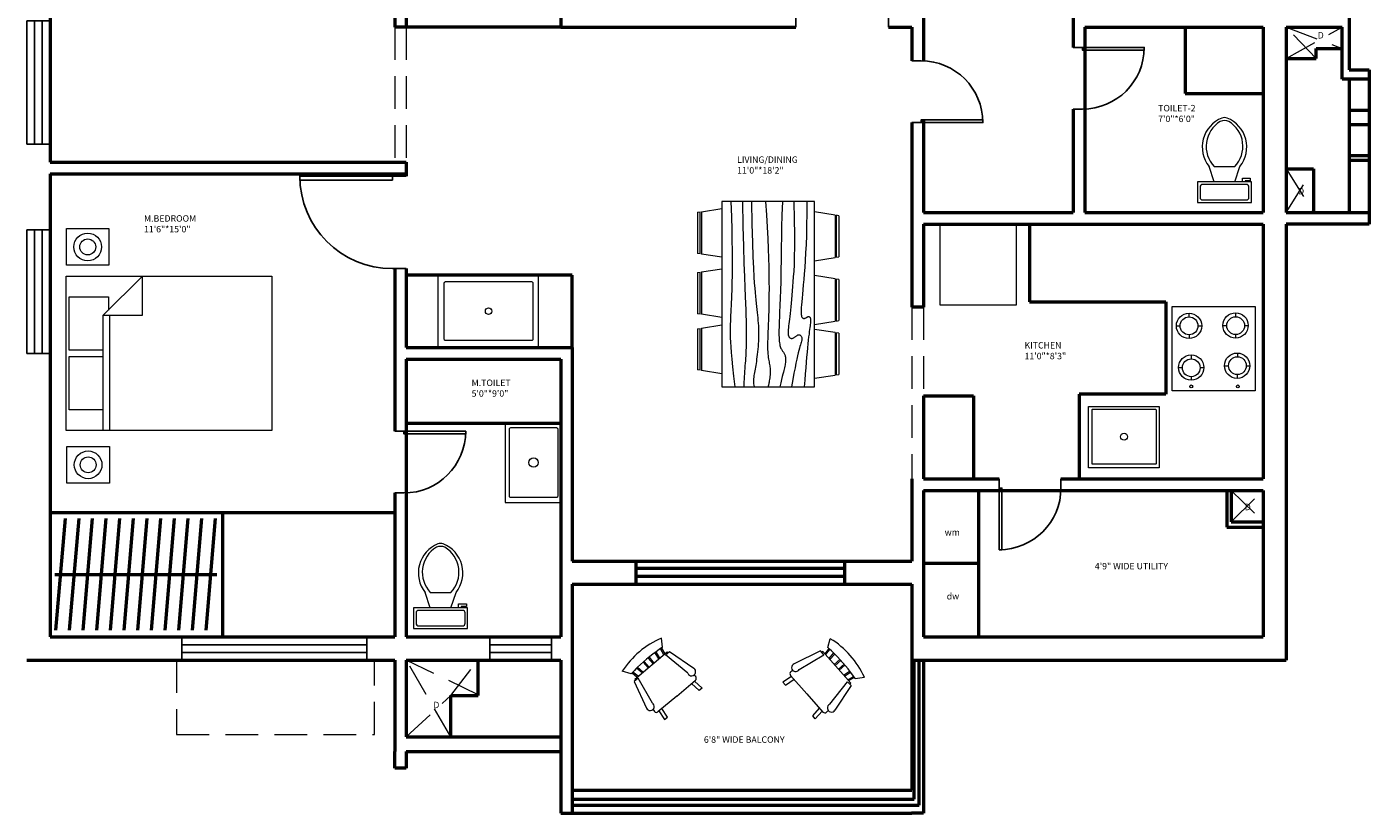
# Model space of a CAD drawing. Units: inches. Extents: x 291 to 2631, y 456 to 2623.
# Tile 10 of 22: x 2109 to 2631, y 468 to 774. Entities that reach past the tile are written whole.
import ezdxf

# ---------------------------------------------------------------- set-up
doc = ezdxf.new("R2010")
doc.units = ezdxf.units.IN
doc.linetypes.add('DASHED', pattern=[19.05, 12.7, -6.35])
for name, color, linetype, lineweight in [('A-ANNO-TEXT', 3, 'Continuous', 25), ('A-AREA-IDEN', 7, 'Continuous', 25), ('A-DOOR', 3, 'Continuous', 25), ('A-EQPM', 8, 'Continuous', 18), ('A-FLOR-FIXT', 9, 'Continuous', 18), ('A-FLOR-OVHD', 1, 'DASHED', 18), ('A-FURN', 8, 'Continuous', 18), ('A-GLAZ', 4, 'Continuous', 25), ('A-WALL', 7, 'Continuous', 50)]:
    doc.layers.add(name, color=color, linetype=linetype, lineweight=lineweight)
doc.styles.get("Standard").update_dxf_attribs({"font": 'arial.ttf'})

# ---------------------------------------------------------------- blocks, each defined once
blk = doc.blocks.new('*U2')
for p, q in [((0, 0), (0, -6)), ((40, 0), (40, -6))]:
    blk.add_line(p, q)
blk.add_lwpolyline([(0, 0), (0, 40), (1.75, 40), (1.75, 0)], close=True)
blk.add_arc((0, 0), 40, 0, 90)
blk = doc.blocks.new('Toilet - top')
for p, q in [((9.5, -6), (9.5, -2)), ((-10, -8.5), (-8, -8.5)), ((-10, -9.5), (-10, -8.5)), ((-7, -9.5), (-10, -9.5)), ((-8, -8.5), (-8, -8)), ((-7, -8), (-7, -9.5)), ((-4, -8), (-6, -14)), ((4, -8), (6, -14)), ((4, -14), (-4, -14))]:
    blk.add_line(p, q)
blk.add_lwpolyline([(10.5, -8), (10.5, 0), (-10.5, 0), (-10.5, -8)], close=True)
for points in [[(-9.5, -2), (-9.5, -6)], [(8.5, -1), (-8.5, -1)], [(-8.5, -7), (8.5, -7)]]:
    blk.add_lwpolyline(points)
for centre, radius, start, end in [((-8.62, -1.88), 0.884, 81.8699, 188.1301), ((8.62, -1.88), 0.884, 351.8699, 98.1301), ((-8.62, -6.12), 0.884, 171.8699, 278.1301), ((8.62, -6.12), 0.884, 261.8699, 8.1301), ((3.52, -21.58), 12.17, 141.4691, 247.9714), ((4.2, -21.82), 11.33, 136.3677, 238.9468), ((-3.52, -21.58), 12.17, 292.0284, 38.5307), ((-4.2, -21.82), 11.33, 301.053, 43.6321), ((0, -27.88), 4, 245.7318, 294.2682), ((0, -29), 4, 254.8605, 285.1395)]:
    blk.add_arc(centre, radius, start, end)
blk = doc.blocks.new('Bed - Queen')
for p, q in [((0, -80.00003), (0, 0)), ((0, 0), (59.99999, 0)), ((59.99999, 0), (59.99999, -80.00003)), ((7.99999, -1.2), (28.79998, -1.2)), ((7.99999, -14.4), (7.99999, -1.2)), ((28.79998, -1.2), (28.79998, -14.4)), ((31.19999, -1.2), (51.99999, -1.2)), ((31.19999, -14.4), (31.19999, -1.2)), ((51.99999, -1.2), (51.99999, -16.4)), ((0, -14.4), (44.8, -14.4)), ((59.99999, -29.6), (44.8, -14.4)), ((44.8, -14.4), (44.8, -29.6)), ((44.8, -16.8), (0, -16.8)), ((51.99999, -16.4), (46.79936, -16.4)), ((44.8, -29.6), (59.99999, -29.6)), ((59.99999, -80.00003), (0, -80.00003))]:
    blk.add_line(p, q)
blk = doc.blocks.new('Chair - Rocking')
for p, q in [((-8, -4.5), (-10, -1.5)), ((-7.5, -4.5), (-7, -7)), ((-6.5, -7), (-7.02225, -4.43)), ((-4.5, -7), (-4.96674, -4.19951)), ((-4, -7), (-4.40532, -4.16272)), ((-1.5, -4.05012), (-1.5, -7)), ((-1, -7), (-1, -4.05012)), ((1, -7), (1, -4.04655)), ((1.5, -4.05012), (1.5, -7)), ((4, -7), (4.40187, -4.18694)), ((4.5, -7), (4.96761, -4.19437)), ((6.5, -7), (7, -4.4057)), ((7.5, -4.5), (7, -7)), ((8, -4.5), (10, -1.5)), ((-9, -7.5), (-12, -18.49999)), ((-7, -7.5), (-9, -7.5)), ((-9, -18.49999), (-7, -7.5)), ((-8.23428, -6.99939), (-8.3093, -7.47958)), ((-8.23041, -7), (8.23915, -7)), ((7, -7.5), (9, -7.5)), ((9, -18.49999), (7, -7.5)), ((8.31071, -7.48854), (8.23449, -7.00073)), ((9, -7.5), (12, -18.49999)), ((-10.36644, -20.64523), (-10.5, -21.49999)), ((10.5, -21.49999), (10.3575, -20.58798)), ((-9, -22.49999), (-9.5, -26.49999)), ((0, -22.49999), (-9.5, -22.49999)), ((-8, -26.49999), (-7.5, -22.49999)), ((0, -22.49999), (9.5, -22.49999)), ((8, -26.49999), (7.5, -22.49999)), ((9, -22.49999), (9.5, -26.49999)), ((-9.5, -26.49999), (-8, -26.49999)), ((9.5, -26.49999), (8, -26.49999))]:
    blk.add_line(p, q)
for centre, radius, start, end in [((0, -34.08333), 34.08333, 72.93847, 107.0615), ((0, -68.25004), 64.25, 93.92211, 97.15267), ((0, -68.25004), 64.25, 82.84733, 93.92211), ((-10.5, -18.99999), 1.58114, 161.5651, 18.43495), ((10.5, -18.99999), 1.58114, 161.5651, 18.43495), ((-9.5, -21.49999), 1, 180, 270), ((9.5, -21.49999), 1, 270, 0)]:
    blk.add_arc(centre, radius, start, end)
blk = doc.blocks.new('WIN-1800')
for p, q in [((0, 9), (72, 9)), ((0, 0), (0, 9)), ((0, 6), (72, 6)), ((72, 9), (72, 0)), ((72, 3), (0, 3)), ((72, 0), (0, 0))]:
    blk.add_line(p, q)
blk = doc.blocks.new('WIN-1200')
for p, q in [((0, 0), (0, 48)), ((0, 48), (9, 48)), ((3, 0), (3, 48)), ((6, 48), (6, 0)), ((9, 48), (9, 0)), ((9, 0), (0, 0))]:
    blk.add_line(p, q)
blk = doc.blocks.new('COOKTOP')
for p, q in [((6.54, 28.68), (6.54, 30.14)), ((24.62, 30.31), (24.62, 28.76)), ((1.62, 25.22), (3.08, 25.22)), ((6.54, 21.76), (6.54, 20.3)), ((10, 25.22), (11.46, 25.22)), ((19.7, 25.39), (21.21, 25.39)), ((24.62, 21.83), (24.62, 20.47)), ((28.13, 25.39), (29.54, 25.39)), ((7.38, 13.92), (7.38, 12.38)), ((25.35, 14.65), (25.34, 13.21)), ((2.46, 9), (3.95, 9)), ((7.38, 5.46), (7.38, 4.08)), ((10.87, 9), (12.3, 9)), ((20.32, 9.73), (21.89, 9.73)), ((25.26, 6.28), (25.24, 4.81)), ((28.81, 9.73), (30.16, 9.73))]:
    blk.add_line(p, q)
blk.add_lwpolyline([(0, 32.79), (32.25, 32.79), (32.25, 0), (0, 0)], close=True)
for centre, radius in [((6.54, 25.22), 4.92), ((6.54, 25.22), 3.46), ((24.62, 25.39), 4.92), ((24.67, 25.29), 3.46), ((7.38, 9), 4.92), ((7.41, 8.92), 3.46), ((25.24, 9.73), 4.92), ((25.35, 9.74), 3.46), ((7.38, 1.69), 0.572), ((25.5, 1.69), 0.572)]:
    blk.add_circle(centre, radius)
blk = doc.blocks.new('WIN-600')
for p, q in [((24, 9), (0, 9)), ((0, 9), (0, 0)), ((24, 6), (0, 6)), ((24, 0), (24, 9)), ((0, 3), (24, 3)), ((0, 0), (24, 0))]:
    blk.add_line(p, q)

msp = doc.modelspace()

# ---------------------------------------------------------------- linework, layer by layer
at = {"layer": 'A-FLOR-OVHD'}
for p, q in [((2251.97, 773.48), (2251.97, 720.98)), ((2256.47, 773.48), (2256.47, 720.98)), ((2598.47, 773.48), (2620.18, 765.26)), ((2598.47, 761.4), (2620.18, 773.48)), ((2610.19, 761.4), (2598.47, 773.48)), ((2598.47, 718.48), (2609.11, 701.48)), ((2598.47, 701.48), (2609.11, 718.48)), ((2452.97, 664.67), (2452.97, 597.98)), ((2457.47, 664.67), (2457.47, 630.2)), ((2577.06, 593.48), (2589.47, 581.26)), ((2577.06, 581.26), (2589.47, 593.48)), ((2167.17, 527.48), (2167.17, 498.51)), ((2244.14, 498.51), (2244.14, 527.48)), ((2273.76, 497.61), (2256.47, 527.48)), ((2284.38, 514), (2256.47, 527.48)), ((2273.76, 513.73), (2284.38, 527.48)), ((2256.47, 497.61), (2273.76, 513.73)), ((2167.17, 498.51), (2244.14, 498.51))]:
    msp.add_line(p, q, dxfattribs=at)
at = {"layer": 'A-FURN'}
for p, q in [((2379.15, 705.74), (2379.15, 633.74)), ((2415.15, 705.74), (2379.15, 705.74)), ((2415.15, 633.74), (2415.15, 705.74)), ((2369.65, 701.56), (2370.65, 701.71)), ((2369.65, 701.56), (2369.65, 685.56)), ((2370.65, 685.4), (2370.65, 701.71)), ((2371.15, 701.79), (2379.15, 703.04)), ((2371.15, 701.79), (2371.15, 685.32)), ((2423.15, 700.46), (2415.15, 701.71)), ((2423.15, 700.45), (2423.15, 683.98)), ((2424.65, 700.22), (2423.65, 700.38)), ((2423.65, 684.06), (2423.65, 700.37)), ((2424.65, 700.22), (2424.65, 684.22)), ((2370.65, 685.4), (2369.65, 685.56)), ((2379.15, 684.07), (2371.15, 685.32)), ((2415.15, 682.74), (2423.15, 683.99)), ((2423.65, 684.07), (2424.65, 684.22)), ((2369.65, 678.15), (2370.65, 678.3)), ((2370.65, 661.99), (2370.65, 678.3)), ((2371.15, 678.38), (2379.15, 679.63)), ((2371.15, 678.38), (2371.15, 661.91)), ((2369.65, 678.15), (2369.65, 662.15)), ((2423.15, 675.68), (2415.15, 676.93)), ((2423.15, 675.67), (2423.15, 659.2)), ((2424.65, 675.44), (2423.65, 675.6)), ((2423.65, 659.28), (2423.65, 675.59)), ((2424.65, 675.44), (2424.65, 659.44)), ((2370.65, 661.99), (2369.65, 662.15)), ((2379.15, 660.66), (2371.15, 661.91)), ((2371.15, 656.53), (2379.15, 657.78)), ((2415.15, 657.96), (2423.15, 659.21)), ((2423.65, 659.28), (2424.65, 659.44)), ((2369.65, 656.3), (2370.65, 656.45)), ((2369.65, 656.3), (2369.65, 640.3)), ((2370.65, 640.14), (2370.65, 656.45)), ((2371.15, 656.53), (2371.15, 640.06)), ((2423.15, 654.77), (2415.15, 656.02)), ((2423.15, 654.77), (2423.15, 638.3)), ((2424.65, 654.54), (2423.65, 654.69)), ((2423.65, 638.38), (2423.65, 654.69)), ((2424.65, 654.54), (2424.65, 638.54)), ((2370.65, 640.14), (2369.65, 640.3)), ((2379.15, 638.81), (2371.15, 640.06)), ((2415.15, 637.05), (2423.15, 638.3)), ((2423.65, 638.38), (2424.65, 638.54)), ((2379.15, 633.74), (2415.15, 633.74))]:
    msp.add_line(p, q, dxfattribs=at)
for points in [[(2382.65, 705.74), (2382.82, 699.83), (2382.94, 694.78), (2383.02, 690.48), (2383.08, 686.82), (2383.1, 683.71), (2383.11, 681.05), (2383.09, 678.72), (2383.07, 676.62), (2383.03, 674.67), (2382.99, 672.84), (2382.94, 671.12), (2382.89, 669.5), (2382.83, 667.98), (2382.78, 666.55), (2382.71, 665.19), (2382.65, 663.91), (2382.59, 662.69), (2382.53, 661.51), (2382.47, 660.35), (2382.43, 659.2), (2382.39, 658.03), (2382.36, 656.82), (2382.35, 655.55), (2382.36, 654.2), (2382.39, 652.75), (2382.45, 651.13), (2382.55, 649.26), (2382.71, 647.08), (2382.94, 644.51), (2383.24, 641.48), (2383.65, 637.92), (2384.15, 633.74)], [(2387.15, 705.74), (2387.34, 696.15), (2387.52, 688.21), (2387.7, 681.73), (2387.87, 676.48), (2388.03, 672.27), (2388.17, 668.87), (2388.3, 666.07), (2388.4, 663.66), (2388.48, 661.47), (2388.54, 659.44), (2388.59, 657.57), (2388.61, 655.85), (2388.62, 654.26), (2388.61, 652.79), (2388.59, 651.42), (2388.57, 650.16), (2388.53, 648.98), (2388.49, 647.88), (2388.44, 646.83), (2388.39, 645.82), (2388.32, 644.84), (2388.26, 643.87), (2388.19, 642.9), (2388.11, 641.91), (2388.03, 640.9), (2387.95, 639.86), (2387.87, 638.81), (2387.8, 637.77), (2387.74, 636.72), (2387.69, 635.7), (2387.66, 634.7), (2387.65, 633.74)], [(2390.65, 705.74), (2390.84, 696.93), (2391.03, 689.83), (2391.21, 684.21), (2391.39, 679.85), (2391.57, 676.52), (2391.74, 673.98), (2391.91, 672.01), (2392.07, 670.37), (2392.22, 668.87), (2392.36, 667.47), (2392.5, 666.16), (2392.63, 664.92), (2392.75, 663.74), (2392.86, 662.62), (2392.97, 661.54), (2393.07, 660.49), (2393.16, 659.47), (2393.24, 658.47), (2393.31, 657.48), (2393.36, 656.49), (2393.4, 655.51), (2393.42, 654.52), (2393.42, 653.52), (2393.4, 652.49), (2393.36, 651.45), (2393.3, 650.4), (2393.22, 649.34), (2393.12, 648.3), (2393.01, 647.27), (2392.9, 646.27), (2392.78, 645.32), (2392.65, 644.41), (2392.53, 643.57), (2392.4, 642.78), (2392.28, 642.03), (2392.16, 641.32), (2392.04, 640.64), (2391.92, 639.99), (2391.8, 639.34), (2391.69, 638.7), (2391.59, 638.06), (2391.49, 637.42), (2391.42, 636.78), (2391.38, 636.15), (2391.37, 635.52), (2391.41, 634.91), (2391.5, 634.32), (2391.65, 633.74)], [(2396.15, 705.74), (2396.49, 700.54), (2396.77, 695.76), (2396.99, 691.4), (2397.16, 687.4), (2397.28, 683.75), (2397.36, 680.4), (2397.42, 677.32), (2397.44, 674.49), (2397.45, 671.88), (2397.44, 669.46), (2397.41, 667.21), (2397.38, 665.13), (2397.33, 663.19), (2397.27, 661.38), (2397.21, 659.68), (2397.15, 658.08), (2397.09, 656.55), (2397.03, 655.11), (2396.98, 653.75), (2396.93, 652.46), (2396.9, 651.26), (2396.88, 650.14), (2396.88, 649.11), (2396.9, 648.16), (2396.94, 647.3), (2397.01, 646.51), (2397.08, 645.79), (2397.17, 645.13), (2397.27, 644.52), (2397.37, 643.95), (2397.47, 643.42), (2397.57, 642.91), (2397.66, 642.42), (2397.74, 641.93), (2397.81, 641.46), (2397.86, 640.97), (2397.9, 640.48), (2397.92, 639.98), (2397.92, 639.46), (2397.9, 638.91), (2397.86, 638.34), (2397.8, 637.75), (2397.72, 637.16), (2397.64, 636.58), (2397.55, 636.04), (2397.47, 635.55), (2397.39, 635.13), (2397.32, 634.79), (2397.26, 634.53), (2397.22, 634.36), (2397.19, 634.24), (2397.17, 634.16), (2397.16, 634.09), (2397.15, 634.01), (2397.15, 633.9), (2397.15, 633.74)], [(2402.65, 705.74), (2402.49, 700.46), (2402.36, 695.81), (2402.27, 691.74), (2402.2, 688.17), (2402.16, 685.05), (2402.12, 682.3), (2402.1, 679.86), (2402.07, 677.66), (2402.03, 675.65), (2401.99, 673.8), (2401.94, 672.09), (2401.89, 670.48), (2401.83, 668.97), (2401.78, 667.52), (2401.71, 666.12), (2401.65, 664.74), (2401.59, 663.37), (2401.53, 662.01), (2401.47, 660.67), (2401.42, 659.37), (2401.38, 658.11), (2401.35, 656.92), (2401.33, 655.79), (2401.32, 654.74), (2401.33, 653.79), (2401.35, 652.93), (2401.39, 652.14), (2401.44, 651.44), (2401.51, 650.81), (2401.6, 650.26), (2401.7, 649.76), (2401.82, 649.33), (2401.95, 648.95), (2402.1, 648.61), (2402.25, 648.32), (2402.41, 648.06), (2402.58, 647.82), (2402.74, 647.59), (2402.91, 647.38), (2403.07, 647.16), (2403.22, 646.94), (2403.36, 646.7), (2403.49, 646.46), (2403.61, 646.19), (2403.71, 645.91), (2403.79, 645.6), (2403.86, 645.27), (2403.9, 644.91), (2403.92, 644.52), (2403.92, 644.1), (2403.89, 643.66), (2403.85, 643.19), (2403.78, 642.71), (2403.7, 642.2), (2403.6, 641.69), (2403.48, 641.16), (2403.35, 640.62), (2403.2, 640.04), (2403.02, 639.38), (2402.82, 638.61), (2402.58, 637.7), (2402.31, 636.6), (2402, 635.3), (2401.65, 633.74)], [(2407.15, 705.74), (2407.29, 698.72), (2407.36, 692.92), (2407.35, 688.17), (2407.29, 684.31), (2407.18, 681.18), (2407.05, 678.62), (2406.89, 676.46), (2406.73, 674.54), (2406.58, 672.71), (2406.44, 670.97), (2406.3, 669.3), (2406.16, 667.72), (2406.03, 666.22), (2405.9, 664.8), (2405.78, 663.48), (2405.65, 662.24), (2405.53, 661.1), (2405.41, 660.05), (2405.29, 659.09), (2405.18, 658.21), (2405.09, 657.42), (2405.01, 656.7), (2404.94, 656.06), (2404.9, 655.49), (2404.88, 655), (2404.88, 654.56), (2404.91, 654.19), (2404.95, 653.87), (2405.02, 653.6), (2405.1, 653.36), (2405.2, 653.16), (2405.32, 652.99), (2405.45, 652.85), (2405.6, 652.73), (2405.75, 652.64), (2405.92, 652.57), (2406.1, 652.53), (2406.28, 652.51), (2406.46, 652.53), (2406.65, 652.58), (2406.84, 652.66), (2407.03, 652.76), (2407.21, 652.88), (2407.4, 653.02), (2407.59, 653.16), (2407.78, 653.3), (2407.96, 653.45), (2408.15, 653.58), (2408.34, 653.69), (2408.53, 653.79), (2408.71, 653.87), (2408.89, 653.92), (2409.07, 653.95), (2409.24, 653.94), (2409.41, 653.9), (2409.57, 653.83), (2409.72, 653.72), (2409.86, 653.57), (2409.98, 653.38), (2410.09, 653.17), (2410.17, 652.93), (2410.22, 652.67), (2410.25, 652.38), (2410.23, 652.08), (2410.18, 651.76), (2410.1, 651.4), (2409.98, 651.01), (2409.83, 650.55), (2409.66, 650.03), (2409.47, 649.41), (2409.25, 648.7), (2409.03, 647.87), (2408.78, 646.91), (2408.52, 645.79), (2408.24, 644.47), (2407.92, 642.92), (2407.56, 641.1), (2407.15, 638.99), (2406.68, 636.55), (2406.15, 633.74)], [(2412.15, 705.74), (2412.13, 700.92), (2412.07, 696.55), (2411.97, 692.6), (2411.84, 689.02), (2411.69, 685.78), (2411.52, 682.84), (2411.34, 680.16), (2411.15, 677.7), (2410.96, 675.43), (2410.78, 673.35), (2410.61, 671.44), (2410.44, 669.71), (2410.3, 668.15), (2410.17, 666.76), (2410.06, 665.55), (2409.98, 664.49), (2409.94, 663.61), (2409.92, 662.86), (2409.93, 662.26), (2409.96, 661.77), (2410.02, 661.38), (2410.1, 661.07), (2410.2, 660.84), (2410.32, 660.66), (2410.45, 660.52), (2410.6, 660.42), (2410.75, 660.36), (2410.91, 660.32), (2411.08, 660.31), (2411.24, 660.32), (2411.41, 660.36), (2411.57, 660.41), (2411.72, 660.48), (2411.87, 660.56), (2412.01, 660.65), (2412.14, 660.73), (2412.27, 660.82), (2412.4, 660.89), (2412.53, 660.95), (2412.65, 660.99), (2412.78, 661.01), (2412.9, 661.01), (2413.02, 660.98), (2413.13, 660.93), (2413.24, 660.86), (2413.33, 660.76), (2413.41, 660.64), (2413.48, 660.49), (2413.54, 660.33), (2413.58, 660.13), (2413.6, 659.89), (2413.61, 659.62), (2413.6, 659.3), (2413.58, 658.92), (2413.54, 658.49), (2413.48, 657.99), (2413.41, 657.43), (2413.33, 656.78), (2413.23, 656.03), (2413.12, 655.18), (2413, 654.21), (2412.86, 653.1), (2412.72, 651.86), (2412.57, 650.45), (2412.41, 648.89), (2412.24, 647.16), (2412.07, 645.27), (2411.89, 643.24), (2411.71, 641.06), (2411.53, 638.75), (2411.34, 636.31), (2411.15, 633.74)]]:
    msp.add_lwpolyline(points, dxfattribs=at)
for points in [[(2124.4, 695.25), (2140.88, 695.25), (2140.88, 680.95), (2124.4, 680.95)], [(2464.03, 696.98), (2493.54, 696.98), (2493.54, 665.42), (2464.03, 665.42)], [(2268.91, 677.11), (2307.71, 677.11), (2307.71, 648.98), (2268.91, 648.98)], [(2521.67, 626.1), (2549.11, 626.1), (2549.11, 602.2), (2521.67, 602.2)], [(2316.47, 619.55), (2294.95, 619.55), (2294.95, 588.8), (2316.47, 588.8)], [(2124.55, 610.55), (2141.04, 610.55), (2141.04, 596.25), (2124.55, 596.25)]]:
    msp.add_lwpolyline(points, close=True, dxfattribs=at)
for points in [[(2271.72, 674.6), (2305.19, 674.6, -0.414214), (2305.69, 674.1), (2305.69, 652.2, -0.414214), (2305.19, 651.7), (2271.72, 651.7, -0.414214), (2271.22, 652.2), (2271.22, 674.1, -0.414214)], [(2523.31, 624.99), (2547.61, 624.99, -0.414214), (2547.91, 624.69), (2547.91, 603.91, -0.414214), (2547.61, 603.61), (2523.31, 603.61, -0.414214), (2523.01, 603.91), (2523.01, 624.69, -0.414214)], [(2297.06, 617.84), (2314.83, 617.84, -0.414214), (2315.33, 617.34), (2315.33, 591.15, -0.414214), (2314.83, 590.65), (2297.06, 590.65, -0.414214), (2296.56, 591.15), (2296.56, 617.34, -0.414214)]]:
    msp.add_lwpolyline(points, format="xyb", close=True, dxfattribs=at)
for centre, radius in [((2132.64, 688.1), 5.39), ((2132.64, 688.1), 3.08), ((2288.46, 663.15), 1.27), ((2535.46, 614.3), 1.36), ((2132.79, 603.4), 5.39), ((2132.79, 603.4), 3.08), ((2305.94, 604.25), 1.82)]:
    msp.add_circle(centre, radius, dxfattribs=at)
at = {"layer": 'A-WALL'}
for p, q in [((2117.97, 921.98), (2117.97, 720.98)), ((2251.97, 921.98), (2251.97, 773.48)), ((2457.47, 921.98), (2457.47, 773.48)), ((2256.47, 809.48), (2256.47, 773.48)), ((2316.47, 809.48), (2316.47, 773.48)), ((2515.69, 777.98), (2515.69, 765.67)), ((2622.9, 779.28), (2622.9, 756.88)), ((2316.47, 773.48), (2251.97, 773.48)), ((2316.47, 773.48), (2407.89, 773.48)), ((2443.89, 773.48), (2452.97, 773.48)), ((2452.97, 773.48), (2452.97, 760.44)), ((2457.47, 773.48), (2457.47, 760.42)), ((2520.19, 773.48), (2520.19, 701.48)), ((2520.19, 773.48), (2589.47, 773.48)), ((2559.17, 773.48), (2559.17, 747.73)), ((2589.47, 773.48), (2589.47, 701.48)), ((2598.47, 773.48), (2620.18, 773.48)), ((2598.47, 773.48), (2598.47, 701.48)), ((2620.18, 756.88), (2620.18, 773.48)), ((2610.19, 761.4), (2610.19, 765.26)), ((2610.19, 765.26), (2620.18, 765.26)), ((2598.47, 761.4), (2610.19, 761.4)), ((2620.18, 753.26), (2620.18, 756.88)), ((2622.9, 756.88), (2630.73, 756.88)), ((2630.73, 756.88), (2630.73, 753.26)), ((2622.9, 753.26), (2620.18, 753.26)), ((2630.73, 753.26), (2622.9, 753.26)), ((2622.9, 753.26), (2622.9, 701.48)), ((2630.73, 753.26), (2630.73, 696.98)), ((2559.17, 747.73), (2589.47, 747.73)), ((2515.69, 741.67), (2515.69, 701.48)), ((2622.9, 741.23), (2622.9, 741.23)), ((2622.9, 741.23), (2630.73, 741.23)), ((2452.97, 736.44), (2452.97, 664.67)), ((2457.47, 737.49), (2457.47, 701.48)), ((2622.9, 735.75), (2630.73, 735.75)), ((2117.97, 720.98), (2256.47, 720.98)), ((2256.47, 720.98), (2256.47, 715.66)), ((2622.9, 723.68), (2630.73, 723.68)), ((2622.9, 721.88), (2630.73, 721.88)), ((2117.97, 716.48), (2256.47, 716.48)), ((2117.97, 716.48), (2117.97, 536.48)), ((2251.97, 716.48), (2251.97, 715.66)), ((2598.47, 718.48), (2609.11, 718.48)), ((2609.11, 718.48), (2609.11, 701.48)), ((2457.47, 701.48), (2515.69, 701.48)), ((2520.19, 701.48), (2589.47, 701.48)), ((2598.47, 701.48), (2630.73, 701.48)), ((2457.47, 696.98), (2589.47, 696.98)), ((2457.47, 696.98), (2457.47, 664.67)), ((2498.71, 696.98), (2498.71, 666.81)), ((2589.47, 696.98), (2589.47, 597.98)), ((2622.9, 696.98), (2598.47, 696.98)), ((2598.47, 696.98), (2598.47, 527.48)), ((2630.73, 696.98), (2622.9, 696.98)), ((2251.97, 679.66), (2251.97, 616.47)), ((2256.47, 679.66), (2256.47, 648.98)), ((2320.97, 677.11), (2256.47, 677.11)), ((2320.97, 648.98), (2320.97, 677.11)), ((2457.47, 664.67), (2452.97, 664.67)), ((2498.71, 666.81), (2551.69, 666.81)), ((2551.69, 666.81), (2551.69, 630.86)), ((2256.47, 648.98), (2320.97, 648.98)), ((2320.97, 648.98), (2320.97, 565.99)), ((2256.47, 644.48), (2316.47, 644.48)), ((2256.47, 644.48), (2256.47, 536.48)), ((2316.47, 644.48), (2316.47, 536.48)), ((2457.47, 630.2), (2476.96, 630.2)), ((2457.47, 630.2), (2457.47, 597.98)), ((2476.96, 630.2), (2476.96, 597.98)), ((2551.69, 630.86), (2518.04, 630.86)), ((2518.04, 630.86), (2518.04, 597.98)), ((2256.47, 619.55), (2316.47, 619.55)), ((2452.97, 597.98), (2452.97, 565.99)), ((2457.47, 597.98), (2486.93, 597.98)), ((2510.93, 597.98), (2589.47, 597.98)), ((2251.97, 592.47), (2251.97, 536.48)), ((2457.47, 593.48), (2589.47, 593.48)), ((2457.47, 593.48), (2457.47, 536.48)), ((2478.91, 593.48), (2478.91, 536.48)), ((2575.44, 593.48), (2575.44, 579.2)), ((2577.06, 593.48), (2577.06, 581.26)), ((2589.47, 593.48), (2589.47, 536.48)), ((2117.97, 584.82), (2251.97, 584.82)), ((2184.97, 584.82), (2184.97, 536.48)), ((2120.27, 539.07), (2123.94, 582.51)), ((2125.57, 539.07), (2129.25, 582.51)), ((2130.88, 539.07), (2134.55, 582.51)), ((2136.18, 539.07), (2139.86, 582.51)), ((2141.49, 539.07), (2145.16, 582.51)), ((2146.79, 539.07), (2150.47, 582.51)), ((2152.1, 539.07), (2155.77, 582.51)), ((2157.4, 539.07), (2161.07, 582.51)), ((2162.7, 539.07), (2166.38, 582.51)), ((2168.01, 539.07), (2171.68, 582.51)), ((2173.31, 539.07), (2176.99, 582.51)), ((2178.62, 539.07), (2182.29, 582.51)), ((2575.44, 579.2), (2589.47, 579.2)), ((2577.06, 581.26), (2589.47, 581.26)), ((2320.97, 565.99), (2452.97, 565.99)), ((2345.73, 565.99), (2345.73, 556.99)), ((2426.77, 565.99), (2426.77, 556.99)), ((2478.91, 564.98), (2457.47, 564.98)), ((2119.89, 560.79), (2182.88, 560.79)), ((2345.73, 563.21), (2426.77, 563.21)), ((2345.73, 560.06), (2426.77, 560.06)), ((2320.97, 556.99), (2452.97, 556.99)), ((2320.97, 556.99), (2320.97, 527.48)), ((2452.97, 556.99), (2452.97, 527.48)), ((2117.97, 536.48), (2251.97, 536.48)), ((2256.47, 536.48), (2316.47, 536.48)), ((2457.47, 536.48), (2589.47, 536.48)), ((2108.97, 527.48), (2251.97, 527.48)), ((2251.97, 527.48), (2251.97, 491.99)), ((2256.47, 527.48), (2256.47, 497.61)), ((2256.47, 527.48), (2316.47, 527.48)), ((2284.38, 513.73), (2284.38, 527.48)), ((2316.47, 527.48), (2316.47, 467.99)), ((2320.97, 527.48), (2320.97, 467.99)), ((2452.97, 527.48), (2598.47, 527.48)), ((2452.97, 527.48), (2452.97, 476.99)), ((2453.93, 473.47), (2453.93, 527.48)), ((2455.84, 471.16), (2455.84, 527.48)), ((2457.47, 527.48), (2457.47, 467.99)), ((2273.76, 497.61), (2273.76, 513.73)), ((2273.76, 513.73), (2284.38, 513.73)), ((2256.47, 497.61), (2316.47, 497.61)), ((2251.97, 485.44), (2251.97, 491.99)), ((2256.47, 491.99), (2316.47, 491.99)), ((2256.47, 491.99), (2256.47, 485.44)), ((2256.47, 485.44), (2251.97, 485.44)), ((2320.97, 476.99), (2452.97, 476.99)), ((2320.97, 473.47), (2453.93, 473.47)), ((2320.97, 471.16), (2455.84, 471.16)), ((2316.47, 467.99), (2320.97, 467.99)), ((2320.97, 467.99), (2452.97, 467.99)), ((2457.47, 467.99), (2452.83, 467.99))]:
    msp.add_line(p, q, dxfattribs=at)

# ---------------------------------------------------------------- block references
at = {"layer": 'A-DOOR', "xscale": -0.9, "yscale": 0.9, "zscale": 0.9}
msp.add_blockref('*U2', (2443.89, 778.88), dxfattribs=at)
at = {"layer": 'A-DOOR'}
for p, xscale, yscale, zscale, rotation in [((2519.29, 765.67), 0.6, 0.6, 0.6, 270), ((2456.57, 736.44), -0.6, 0.6, 0.6, 270), ((2251.07, 715.66), -0.9, 0.9, 0.9, 90), ((2255.57, 616.47), 0.6, 0.6, 0.6, 270), ((2486.93, 594.38), -0.6, 0.6, 0.6, 180)]:
    msp.add_blockref('*U2', p, dxfattribs=dict(at, xscale=xscale, yscale=yscale, zscale=zscale, rotation=rotation))
at = {"layer": 'A-EQPM'}
msp.add_blockref('COOKTOP', (2554.18, 632.2), dxfattribs=at)
at = {"layer": 'A-FLOR-FIXT', "rotation": 180}
for p in [(2574.52, 705.35), (2269.8, 539.81)]:
    msp.add_blockref('Toilet - top', p, dxfattribs=at)
at = {"layer": 'A-FURN'}
for name, p, rotation in [('Bed - Queen', (2124.26, 616.72), 90), ('Chair - Rocking', (2347.09, 530.75), 40.05477191636604), ('Chair - Rocking', (2429.02, 529.3), 311.3871825917978)]:
    msp.add_blockref(name, p, dxfattribs=dict(at, rotation=rotation))
at = {"layer": 'A-GLAZ', "rotation": 180}
for name, p in [('WIN-1200', (2117.97, 776.04)), ('WIN-1200', (2117.97, 694.72)), ('WIN-600', (2312.89, 536.48))]:
    msp.add_blockref(name, p, dxfattribs=at)
at = {"layer": 'A-GLAZ'}
msp.add_blockref('WIN-1800', (2169.15, 527.48), dxfattribs=at)

# ---------------------------------------------------------------- texts
at = {"layer": 'A-ANNO-TEXT', "char_height": 2.5, "attachment_point": 1}
for s, width, insert in [('D', 1.657, (2610.74, 771.61)), ('D', 2.1307, (2603.12, 711.05)), ('D', 2.108, (2582.37, 588.25)), ('wm', 14.1748, (2465.74, 578.42)), ('dw', 9.504, (2466.52, 553.56)), ('D', 1.5625, (2266.97, 511.3))]:
    msp.add_mtext_dynamic_manual_height_columns(s, width=width, gutter_width=12.5, heights=[0], dxfattribs=dict(at, insert=insert))
at = {"layer": 'A-AREA-IDEN', "char_height": 2.5, "attachment_point": 1}
for s, width, insert in [('TOILET-2\\P7\'0"*6\'0"', 25.6449, (2548.71, 743.3)), ('LIVING/DINING\\P11\'0"*18\'2"', 74.6205, (2385.05, 723.28)), ('M.BEDROOM\\P11\'6"*15\'0"', 52.6992, (2154.5, 700.42)), ('KITCHEN\\P11\'0"*8\'3"', 43.9919, (2496.76, 651.1)), ('M.TOILET\\P5\'0"*9\'0"', 45.7217, (2281.85, 636.54)), ('4\'9" WIDE UTILITY', 71.4063, (2524.1, 565.25)), ('6\'8" WIDE BALCONY', 75.8844, (2372.13, 497.84))]:
    msp.add_mtext_dynamic_manual_height_columns(s, width=width, gutter_width=12.5, heights=[0], dxfattribs=dict(at, insert=insert))

doc.saveas('drawing.dxf')
